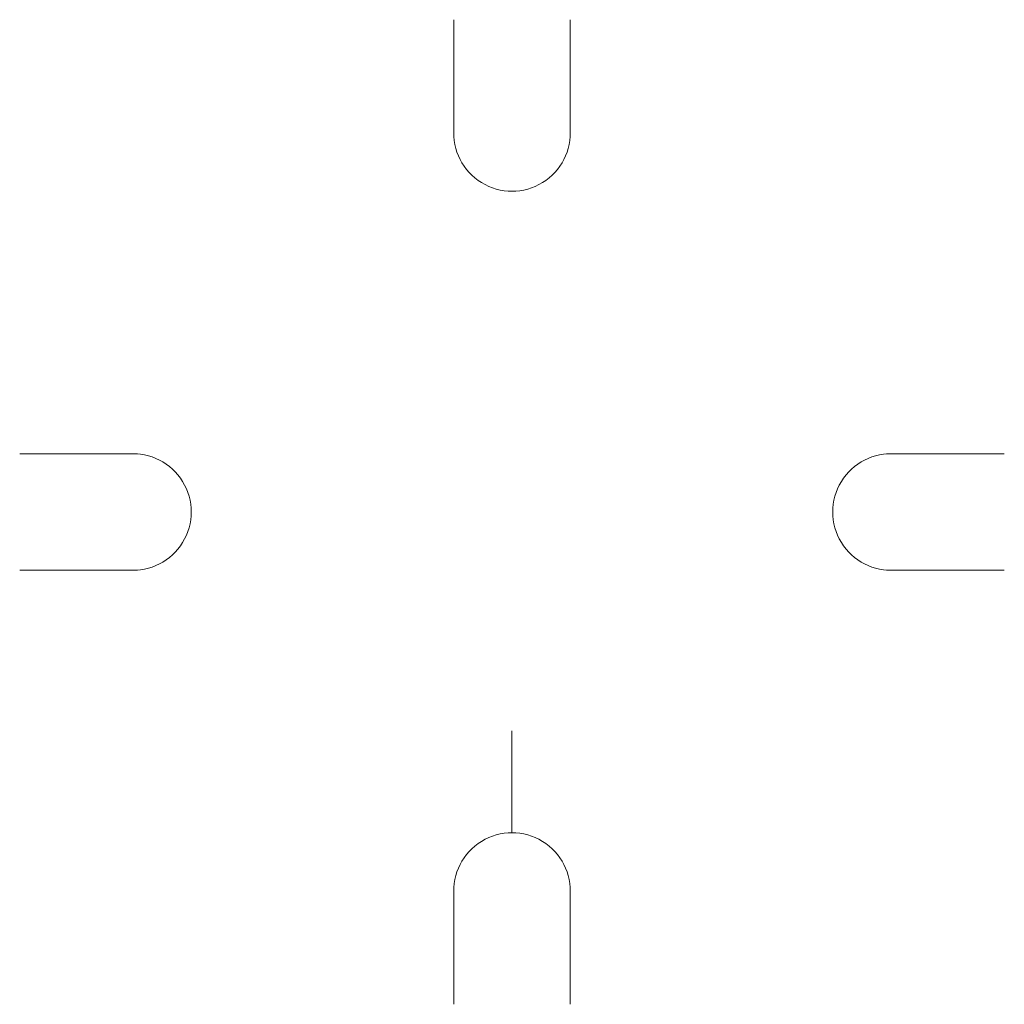
# Model space of a CAD drawing. Units: millimetres. Extents: x 2698.5 to 2766.1, y 1135.2 to 1202.7.
import ezdxf

# ---------------------------------------------------------------- set-up
doc = ezdxf.new("R2010")
doc.units = ezdxf.units.MM
doc.layers.add('M-CONS', color=8, linetype='Continuous', lineweight=13)

msp = doc.modelspace()

# ---------------------------------------------------------------- linework, layer by layer
at = {"layer": 'M-CONS'}
for p, q in [((2728.313, 1194.644), (2728.313, 1202.717)), ((2736.289, 1194.644), (2736.289, 1202.717)), ((2706.609, 1172.94), (2698.536, 1172.94)), ((2757.993, 1172.94), (2766.066, 1172.94)), ((2706.609, 1164.963), (2698.536, 1164.963)), ((2757.993, 1164.963), (2766.066, 1164.963)), ((2732.301, 1146.952), (2732.301, 1153.952)), ((2728.313, 1143.259), (2728.313, 1135.186)), ((2736.289, 1143.259), (2736.289, 1135.186))]:
    msp.add_line(p, q, dxfattribs=at)
for centre, start, end in [((2732.301, 1194.952), 175.58827, 4.41173), ((2706.301, 1168.952), 265.58827, 94.41173), ((2758.301, 1168.952), 85.58827, 274.41173), ((2732.301, 1142.952), 355.58827, 184.41173)]:
    msp.add_arc(centre, 4, start, end, dxfattribs=at)

doc.saveas('drawing.dxf')
